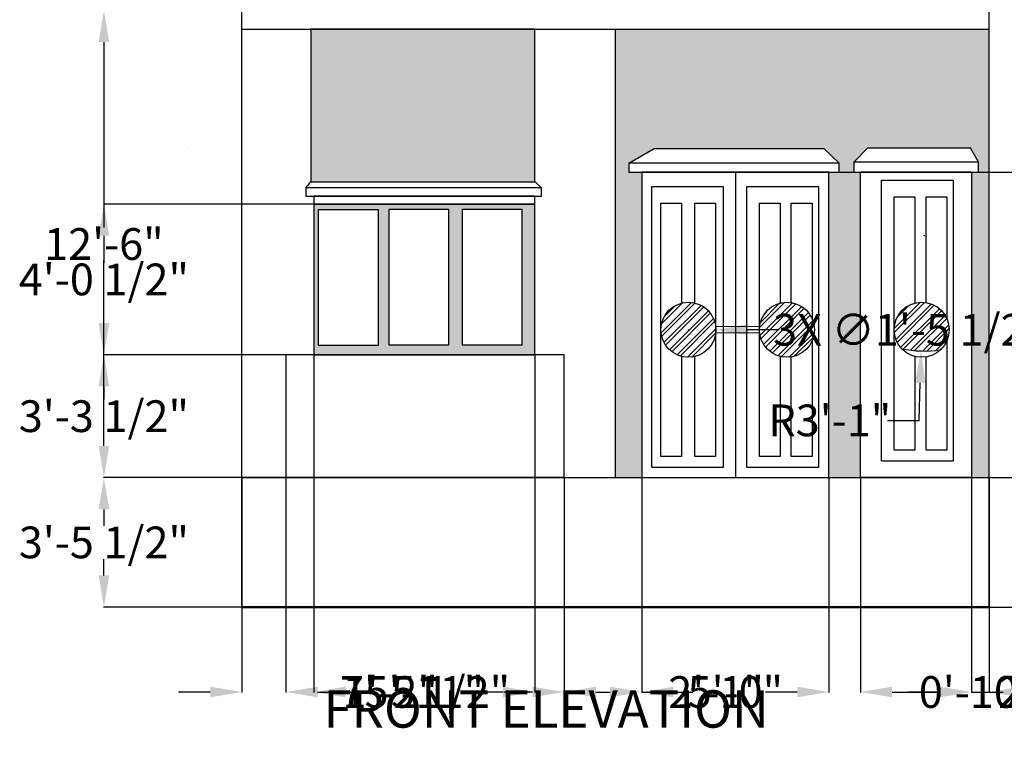
# Model space of a CAD drawing. Units: inches. Extents: x 21 to 3450, y 4 to 2137.
# Tile 5 of 14: x 2115 to 2431, y 1552 to 1783. Entities that reach past the tile are written whole.
import ezdxf

# ---------------------------------------------------------------- set-up
doc = ezdxf.new("R2010")
doc.units = ezdxf.units.IN
doc.header["$MEASUREMENT"] = 0
for name, color, linetype, lineweight in [('A-ANNO-DIMS', 2, 'Continuous', 18), ('A-ANNO-TEXT', 7, 'Continuous', 18), ('A-ELEV', 7, 'Continuous', 25), ('A-ELEV-PATT', 8, 'Continuous', 13), ('A-WALL', 7, 'Continuous', 50)]:
    doc.layers.add(name, color=color, linetype=linetype, lineweight=lineweight)
doc.styles.get("Standard").update_dxf_attribs({"font": 'arial.ttf'})
doc.dimstyles.get("Standard").update_dxf_attribs({"dimtxt": 10.18, "dimasz": 10.18, "dimexe": 0.18, "dimexo": 0.0625, "dimgap": 0.09, "dimtad": 0, "dimtih": 1, "dimtoh": 1, "dimdec": 0, "dimzin": 0, "dimdsep": 46, "dimlunit": 3, "dimtxsty": 'Standard', "dimcen": 0.09, "dimadec": 0, "dimazin": 0, "dimtfac": 1, "dimtdec": 0, "dimtofl": 0, "dimtmove": 0, "dimatfit": 3, "dimfxl": 1, "dimtolj": 1, "dimtzin": 0, "dimarcsym": 0})
pattern_1 = [(45, (255.9994, -6.4862), (-2.0417708, 2.0417708), []), (45, (257.3606, -6.4862), (-2.0417708, 2.0417708), [])]

# ---------------------------------------------------------------- blocks, each defined once
blk = doc.blocks.new('*D152')
at = {"layer": 'A-ANNO-DIMS', "color": 0, "lineweight": -2, "transparency": 16777216}
for p, q in [((2426.25, 2094.9), (2453.61, 2094.9)), ((2453.43, 2084.72), (2453.43, 1850.06)), ((2453.43, 1604.7), (2453.43, 1839.36)), ((2426.25, 1594.52), (2453.61, 1594.52))]:
    blk.add_line(p, q, dxfattribs=at)
at = {"layer": 'A-ANNO-DIMS', "color": 0, "transparency": 16777216}
for points in [[(2451.74, 2084.72), (2455.13, 2084.72), (2453.43, 2094.9)], [(2451.74, 1604.7), (2455.13, 1604.7), (2453.43, 1594.52)]]:
    blk.add_solid(points, dxfattribs=at)
at = {"layer": 'Defpoints', "color": 0, "transparency": 16777216}
for p in [(2426.18, 2094.9), (2453.43, 2094.9), (2426.18, 1594.52)]:
    blk.add_point(p, dxfattribs=at)
at = {"layer": 'A-ANNO-DIMS', "color": 0, "transparency": 16777216, "insert": (2453.43, 1844.71), "char_height": 10.18, "attachment_point": 5}
blk.add_mtext('\\A1;41\'-8 1/2"', dxfattribs=at)
blk = doc.blocks.new('*D153')
at = {"layer": 'A-ANNO-DIMS', "color": 0, "lineweight": -2, "transparency": 16777216}
for p, q in [((2186.12, 1636.08), (2141.7, 1636.08)), ((2141.88, 1625.9), (2141.88, 1620.66)), ((2141.88, 1604.7), (2141.88, 1609.94)), ((2186.12, 1594.52), (2141.7, 1594.52))]:
    blk.add_line(p, q, dxfattribs=at)
at = {"layer": 'A-ANNO-DIMS', "color": 0, "transparency": 16777216}
for points in [[(2140.19, 1625.9), (2143.58, 1625.9), (2141.88, 1636.08)], [(2140.19, 1604.7), (2143.58, 1604.7), (2141.88, 1594.52)]]:
    blk.add_solid(points, dxfattribs=at)
at = {"layer": 'Defpoints', "color": 0, "transparency": 16777216}
for p in [(2141.88, 1636.08), (2186.18, 1636.08), (2186.18, 1594.52)]:
    blk.add_point(p, dxfattribs=at)
at = {"layer": 'A-ANNO-DIMS', "color": 0, "transparency": 16777216, "insert": (2141.88, 1615.3), "char_height": 10.18, "attachment_point": 5}
blk.add_mtext('\\A1;3\'-5 1/2"', dxfattribs=at)
blk = doc.blocks.new('*D154')
at = {"layer": 'A-ANNO-DIMS', "color": 0, "lineweight": -2, "transparency": 16777216}
for p, q in [((2186.12, 1786.08), (2141.7, 1786.08)), ((2141.88, 1775.9), (2141.88, 1716.37)), ((2141.88, 1646.26), (2141.88, 1705.79)), ((2186.12, 1636.08), (2141.7, 1636.08))]:
    blk.add_line(p, q, dxfattribs=at)
at = {"layer": 'A-ANNO-DIMS', "color": 0, "transparency": 16777216}
for points in [[(2140.19, 1775.9), (2143.58, 1775.9), (2141.88, 1786.08)], [(2140.19, 1646.26), (2143.58, 1646.26), (2141.88, 1636.08)]]:
    blk.add_solid(points, dxfattribs=at)
at = {"layer": 'Defpoints', "color": 0, "transparency": 16777216}
for p in [(2141.88, 1786.08), (2186.18, 1786.08), (2186.18, 1636.08)]:
    blk.add_point(p, dxfattribs=at)
at = {"layer": 'A-ANNO-DIMS', "color": 0, "transparency": 16777216, "insert": (2141.88, 1711.08), "char_height": 10.18, "attachment_point": 5}
blk.add_mtext('\\A1;12\'-6"', dxfattribs=at)
blk = doc.blocks.new('*D161')
at = {"layer": 'A-ANNO-DIMS', "color": 0, "lineweight": -2, "transparency": 16777216}
for p, q in [((2186.18, 1636.02), (2186.18, 1567.09)), ((2200.32, 1636.02), (2200.32, 1567.09)), ((2176, 1567.27), (2165.82, 1567.27)), ((2210.5, 1567.27), (2220.68, 1567.27))]:
    blk.add_line(p, q, dxfattribs=at)
at = {"layer": 'A-ANNO-DIMS', "color": 0, "transparency": 16777216}
for points in [[(2176, 1568.97), (2176, 1565.57), (2186.18, 1567.27)], [(2210.5, 1568.97), (2210.5, 1565.57), (2200.32, 1567.27)]]:
    blk.add_solid(points, dxfattribs=at)
at = {"layer": 'Defpoints', "color": 0, "transparency": 16777216}
for p in [(2186.18, 1636.08), (2200.32, 1636.08), (2200.32, 1567.27)]:
    blk.add_point(p, dxfattribs=at)
at = {"layer": 'A-ANNO-DIMS', "color": 0, "transparency": 16777216, "insert": (2233.82, 1567.27), "char_height": 10.18, "attachment_point": 5}
blk.add_mtext('\\A1;1\'-2"', dxfattribs=at)
blk = doc.blocks.new('*D162')
at = {"layer": 'A-ANNO-DIMS', "color": 0, "lineweight": -2, "transparency": 16777216}
for p, q in [((2200.32, 1636.02), (2200.32, 1567.09)), ((2289.7, 1636.02), (2289.7, 1567.09)), ((2210.5, 1567.27), (2219.57, 1567.27)), ((2279.52, 1567.27), (2270.45, 1567.27))]:
    blk.add_line(p, q, dxfattribs=at)
at = {"layer": 'A-ANNO-DIMS', "color": 0, "transparency": 16777216}
for points in [[(2210.5, 1568.97), (2210.5, 1565.57), (2200.32, 1567.27)], [(2279.52, 1568.97), (2279.52, 1565.57), (2289.7, 1567.27)]]:
    blk.add_solid(points, dxfattribs=at)
at = {"layer": 'Defpoints', "color": 0, "transparency": 16777216}
for p in [(2200.32, 1636.08), (2289.7, 1636.08), (2289.7, 1567.27)]:
    blk.add_point(p, dxfattribs=at)
at = {"layer": 'A-ANNO-DIMS', "color": 0, "transparency": 16777216, "insert": (2245.01, 1567.27), "char_height": 10.18, "attachment_point": 5}
blk.add_mtext('\\A1;7\'-5 1/2"', dxfattribs=at)
blk = doc.blocks.new('*D163')
at = {"layer": 'A-ANNO-DIMS', "color": 0, "lineweight": -2, "transparency": 16777216}
for p, q in [((2289.7, 1636.02), (2289.7, 1567.09)), ((2314.57, 1636.02), (2314.57, 1567.09)), ((2299.88, 1567.27), (2304.39, 1567.27)), ((2314.57, 1567.27), (2324.75, 1567.27))]:
    blk.add_line(p, q, dxfattribs=at)
at = {"layer": 'A-ANNO-DIMS', "color": 0, "transparency": 16777216}
for points in [[(2299.88, 1568.97), (2299.88, 1565.57), (2289.7, 1567.27)], [(2304.39, 1568.97), (2304.39, 1565.57), (2314.57, 1567.27)]]:
    blk.add_solid(points, dxfattribs=at)
at = {"layer": 'Defpoints', "color": 0, "transparency": 16777216}
for p in [(2289.7, 1636.08), (2314.57, 1636.08), (2314.57, 1567.27)]:
    blk.add_point(p, dxfattribs=at)
at = {"layer": 'A-ANNO-DIMS', "color": 0, "transparency": 16777216, "insert": (2338.46, 1567.27), "char_height": 10.18, "attachment_point": 5}
blk.add_mtext('\\A1;2\'-1"', dxfattribs=at)
blk = doc.blocks.new('*D164')
at = {"layer": 'A-ANNO-DIMS', "color": 0, "lineweight": -2, "transparency": 16777216}
for p, q in [((2314.57, 1636.02), (2314.57, 1567.09)), ((2374.7, 1636.02), (2374.7, 1567.09)), ((2324.75, 1567.27), (2331.02, 1567.27)), ((2364.52, 1567.27), (2358.26, 1567.27))]:
    blk.add_line(p, q, dxfattribs=at)
at = {"layer": 'A-ANNO-DIMS', "color": 0, "transparency": 16777216}
for points in [[(2324.75, 1568.97), (2324.75, 1565.57), (2314.57, 1567.27)], [(2364.52, 1568.97), (2364.52, 1565.57), (2374.7, 1567.27)]]:
    blk.add_solid(points, dxfattribs=at)
at = {"layer": 'Defpoints', "color": 0, "transparency": 16777216}
for p in [(2314.57, 1636.08), (2374.7, 1636.08), (2374.7, 1567.27)]:
    blk.add_point(p, dxfattribs=at)
at = {"layer": 'A-ANNO-DIMS', "color": 0, "transparency": 16777216, "insert": (2344.64, 1567.27), "char_height": 10.18, "attachment_point": 5}
blk.add_mtext('\\A1;5\'-0"', dxfattribs=at)
blk = doc.blocks.new('*D165')
at = {"layer": 'A-ANNO-DIMS', "color": 0, "lineweight": -2, "transparency": 16777216}
for p, q in [((2374.7, 1636.02), (2374.7, 1567.09)), ((2384.8, 1636.02), (2384.8, 1567.09)), ((2364.52, 1567.27), (2354.34, 1567.27)), ((2394.98, 1567.27), (2405.16, 1567.27))]:
    blk.add_line(p, q, dxfattribs=at)
at = {"layer": 'A-ANNO-DIMS', "color": 0, "transparency": 16777216}
for points in [[(2364.52, 1568.97), (2364.52, 1565.57), (2374.7, 1567.27)], [(2394.98, 1568.97), (2394.98, 1565.57), (2384.8, 1567.27)]]:
    blk.add_solid(points, dxfattribs=at)
at = {"layer": 'Defpoints', "color": 0, "transparency": 16777216}
for p in [(2374.7, 1636.08), (2384.8, 1636.08), (2384.8, 1567.27)]:
    blk.add_point(p, dxfattribs=at)
at = {"layer": 'A-ANNO-DIMS', "color": 0, "transparency": 16777216, "insert": (2422.74, 1567.27), "char_height": 10.18, "attachment_point": 5}
blk.add_mtext('\\A1;0\'-10"', dxfattribs=at)
blk = doc.blocks.new('*D166')
at = {"layer": 'A-ANNO-DIMS', "color": 0, "lineweight": -2, "transparency": 16777216}
for p, q in [((2384.8, 1636.02), (2384.8, 1567.09)), ((2420.5, 1636.02), (2420.5, 1567.09)), ((2394.98, 1567.27), (2410.32, 1567.27)), ((2420.5, 1567.27), (2430.68, 1567.27))]:
    blk.add_line(p, q, dxfattribs=at)
at = {"layer": 'A-ANNO-DIMS', "color": 0, "transparency": 16777216}
for points in [[(2394.98, 1568.97), (2394.98, 1565.57), (2384.8, 1567.27)], [(2410.32, 1568.97), (2410.32, 1565.57), (2420.5, 1567.27)]]:
    blk.add_solid(points, dxfattribs=at)
at = {"layer": 'Defpoints', "color": 0, "transparency": 16777216}
for p in [(2384.8, 1636.08), (2420.5, 1636.08), (2420.5, 1567.27)]:
    blk.add_point(p, dxfattribs=at)
at = {"layer": 'A-ANNO-DIMS', "color": 0, "transparency": 16777216, "insert": (2460.2, 1567.27), "char_height": 10.18, "attachment_point": 5}
blk.add_mtext('\\A1;2\'-11 1/2"', dxfattribs=at)
blk = doc.blocks.new('*D167')
at = {"layer": 'A-ANNO-DIMS', "color": 0, "lineweight": -2, "transparency": 16777216}
for p, q in [((2420.5, 1636.02), (2420.5, 1567.09)), ((2426.18, 1636.02), (2426.18, 1567.09)), ((2410.32, 1567.27), (2400.14, 1567.27)), ((2436.36, 1567.27), (2446.54, 1567.27))]:
    blk.add_line(p, q, dxfattribs=at)
at = {"layer": 'A-ANNO-DIMS', "color": 0, "transparency": 16777216}
for points in [[(2410.32, 1568.97), (2410.32, 1565.57), (2420.5, 1567.27)], [(2436.36, 1568.97), (2436.36, 1565.57), (2426.18, 1567.27)]]:
    blk.add_solid(points, dxfattribs=at)
at = {"layer": 'Defpoints', "color": 0, "transparency": 16777216}
for p in [(2420.5, 1636.08), (2426.18, 1636.08), (2426.18, 1567.27)]:
    blk.add_point(p, dxfattribs=at)
at = {"layer": 'A-ANNO-DIMS', "color": 0, "transparency": 16777216, "insert": (2472.03, 1567.27), "char_height": 10.18, "attachment_point": 5}
blk.add_mtext('\\A1;0\'-5 1/2"', dxfattribs=at)
blk = doc.blocks.new('*D168')
at = {"layer": 'A-ANNO-DIMS', "color": 0, "lineweight": -2, "transparency": 16777216}
for p, q in [((2209.28, 1675.48), (2209.28, 1567.09)), ((2280.25, 1675.48), (2280.25, 1567.09)), ((2219.46, 1567.27), (2227.19, 1567.27)), ((2270.07, 1567.27), (2262.34, 1567.27))]:
    blk.add_line(p, q, dxfattribs=at)
at = {"layer": 'A-ANNO-DIMS', "color": 0, "transparency": 16777216}
for points in [[(2219.46, 1568.97), (2219.46, 1565.57), (2209.28, 1567.27)], [(2270.07, 1568.97), (2270.07, 1565.57), (2280.25, 1567.27)]]:
    blk.add_solid(points, dxfattribs=at)
at = {"layer": 'Defpoints', "color": 0, "transparency": 16777216}
for p in [(2209.28, 1675.54), (2280.25, 1675.54), (2280.25, 1567.27)]:
    blk.add_point(p, dxfattribs=at)
at = {"layer": 'A-ANNO-DIMS', "color": 0, "transparency": 16777216, "insert": (2244.76, 1567.27), "char_height": 10.18, "attachment_point": 5}
blk.add_mtext('\\A1;5\'-11"', dxfattribs=at)
blk = doc.blocks.new('*D169')
at = {"layer": 'A-ANNO-DIMS', "color": 0, "lineweight": -2, "transparency": 16777216}
for p, q in [((2280.19, 1723.89), (2141.7, 1723.89)), ((2141.88, 1713.71), (2141.88, 1705.07)), ((2141.88, 1685.72), (2141.88, 1694.36)), ((2280.19, 1675.54), (2141.7, 1675.54))]:
    blk.add_line(p, q, dxfattribs=at)
at = {"layer": 'A-ANNO-DIMS', "color": 0, "transparency": 16777216}
for points in [[(2140.19, 1713.71), (2143.58, 1713.71), (2141.88, 1723.89)], [(2140.19, 1685.72), (2143.58, 1685.72), (2141.88, 1675.54)]]:
    blk.add_solid(points, dxfattribs=at)
at = {"layer": 'Defpoints', "color": 0, "transparency": 16777216}
for p in [(2141.88, 1723.89), (2280.25, 1723.89), (2280.25, 1675.54)]:
    blk.add_point(p, dxfattribs=at)
at = {"layer": 'A-ANNO-DIMS', "color": 0, "transparency": 16777216, "insert": (2141.88, 1699.71), "char_height": 10.18, "attachment_point": 5}
blk.add_mtext('\\A1;4\'-0 1/2"', dxfattribs=at)
blk = doc.blocks.new('*D170')
at = {"layer": 'A-ANNO-DIMS', "color": 0, "lineweight": -2, "transparency": 16777216}
for p, q in [((2289.64, 1675.54), (2141.7, 1675.54)), ((2141.88, 1665.36), (2141.88, 1661.17)), ((2141.88, 1646.26), (2141.88, 1650.45)), ((2289.64, 1636.08), (2141.7, 1636.08))]:
    blk.add_line(p, q, dxfattribs=at)
at = {"layer": 'A-ANNO-DIMS', "color": 0, "transparency": 16777216}
for points in [[(2140.19, 1665.36), (2143.58, 1665.36), (2141.88, 1675.54)], [(2140.19, 1646.26), (2143.58, 1646.26), (2141.88, 1636.08)]]:
    blk.add_solid(points, dxfattribs=at)
at = {"layer": 'Defpoints', "color": 0, "transparency": 16777216}
for p in [(2141.88, 1675.54), (2289.7, 1675.54), (2289.7, 1636.08)]:
    blk.add_point(p, dxfattribs=at)
at = {"layer": 'A-ANNO-DIMS', "color": 0, "transparency": 16777216, "insert": (2141.88, 1655.81), "char_height": 10.18, "attachment_point": 5}
blk.add_mtext('\\A1;3\'-3 1/2"', dxfattribs=at)
blk = doc.blocks.new('*D173')
at = {"layer": 'A-ANNO-DIMS', "color": 0, "lineweight": -2, "transparency": 16777216}
for p, q in [((2374.76, 1734.1), (2453.61, 1734.1)), ((2453.43, 1723.92), (2453.43, 1690.38)), ((2453.43, 1646.26), (2453.43, 1679.8)), ((2374.76, 1636.08), (2453.61, 1636.08))]:
    blk.add_line(p, q, dxfattribs=at)
at = {"layer": 'A-ANNO-DIMS', "color": 0, "transparency": 16777216}
for points in [[(2451.74, 1723.92), (2455.13, 1723.92), (2453.43, 1734.1)], [(2451.74, 1646.26), (2455.13, 1646.26), (2453.43, 1636.08)]]:
    blk.add_solid(points, dxfattribs=at)
at = {"layer": 'Defpoints', "color": 0, "transparency": 16777216}
for p in [(2374.7, 1734.1), (2453.43, 1734.1), (2374.7, 1636.08)]:
    blk.add_point(p, dxfattribs=at)
at = {"layer": 'A-ANNO-DIMS', "color": 0, "transparency": 16777216, "insert": (2453.43, 1685.09), "char_height": 10.18, "attachment_point": 5}
blk.add_mtext('\\A1;8\'-2"', dxfattribs=at)
blk = doc.blocks.new('*D195')
at = {"layer": 'A-ANNO-DIMS', "color": 0, "lineweight": -2, "transparency": 16777216}
for p, q in [((2329.47, 1683.55), (2329.65, 1683.55)), ((2329.56, 1683.46), (2329.56, 1683.64)), ((2358.76, 1683.55), (2348.58, 1683.55))]:
    blk.add_line(p, q, dxfattribs=at)
at = {"layer": 'A-ANNO-DIMS', "color": 0, "transparency": 16777216}
blk.add_solid([(2348.58, 1685.25), (2348.58, 1681.85), (2338.4, 1683.55)], dxfattribs=at)
at = {"layer": 'Defpoints', "color": 0, "transparency": 16777216}
for p in [(2320.73, 1683.55), (2338.4, 1683.55)]:
    blk.add_point(p, dxfattribs=at)
at = {"layer": 'A-ANNO-DIMS', "color": 0, "transparency": 16777216, "insert": (2400.44, 1683.55), "char_height": 10.18, "attachment_point": 5}
blk.add_mtext('\\A1;3X ∅1\'-5 1/2"', dxfattribs=at)
blk = doc.blocks.new('*D196')
at = {"layer": 'A-ANNO-DIMS', "color": 0, "lineweight": -2, "transparency": 16777216}
for p, q in [((2405.24, 1713.84), (2405.42, 1713.84)), ((2405.33, 1713.75), (2405.33, 1713.93)), ((2403.63, 1654.47), (2403.97, 1666.56)), ((2393.45, 1654.47), (2403.63, 1654.47))]:
    blk.add_line(p, q, dxfattribs=at)
at = {"layer": 'A-ANNO-DIMS', "color": 0, "transparency": 16777216}
blk.add_solid([(2402.28, 1666.61), (2405.67, 1666.51), (2404.27, 1676.74)], dxfattribs=at)
at = {"layer": 'Defpoints', "color": 0, "transparency": 16777216}
for p in [(2405.33, 1713.84), (2404.27, 1676.74)]:
    blk.add_point(p, dxfattribs=at)
at = {"layer": 'A-ANNO-DIMS', "color": 0, "transparency": 16777216, "insert": (2374.95, 1654.47), "char_height": 10.18, "attachment_point": 5}
blk.add_mtext('\\A1;R3\'-1"', dxfattribs=at)

msp = doc.modelspace()

# ---------------------------------------------------------------- hatches: boundary and pattern name
at = {"layer": 'A-ELEV-PATT'}
h = msp.add_hatch(dxfattribs=at)
h.set_pattern_fill('AR-BRELM', color=256, scale=1.9)
h.set_pattern_definition([(0, (0, 0), (0, 10.1346), [14.4875, -0.7125]), (0, (0, 4.275), (0, 10.1346), [14.4875, -0.7125]), (0, (3.8, 5.067), (0, 10.1346), [6.8875, -0.7125]), (0, (3.8, 9.342), (0, 10.1346), [6.8875, -0.7125]), (90, (0, 0), (-15.2, 9e-16), [4.275, -5.8596]), (90, (-0.713, 0), (-15.2, 9e-16), [4.275, -5.8596]), (90, (3.8, 5.067), (-7.6, 5e-16), [4.275, -5.8596]), (90, (3.0875, 5.067), (-7.6, 5e-16), [4.275, -5.8596])])
h.paths.add_polyline_path([(2282.59, 1918.08), (2210.89, 1918.08), (2210.89, 1885.65), (2282.59, 1885.65)])
h.paths.add_polyline_path([(2280.2, 1780.08), (2208.3, 1780.08), (2208.3, 1731.04), (2280.2, 1731.04)])
h.paths.add_polyline_path([(2350.36, 1918.08), (2306.18, 1918.08), (2306.18, 1829.6), (2319, 1829.6), (2319, 1875.89), (2350.36, 1875.89)])
h.paths.add_polyline_path([(2426.18, 1780.08), (2306.18, 1780.08), (2306.18, 1636.08), (2314.57, 1636.08), (2314.57, 1734.1), (2310.48, 1734.1), (2310.48, 1737.04), (2318.62, 1741.75), (2373, 1741.75), (2378.02, 1737.04), (2378.02, 1734.1), (2374.7, 1734.1), (2374.7, 1636.08), (2384.8, 1636.08), (2384.8, 1734.1), (2382.71, 1734.1), (2382.71, 1737.37), (2387.22, 1741.92), (2420.14, 1741.92), (2422.71, 1737.37), (2422.71, 1734.1), (2420.5, 1734.1), (2420.5, 1636.08), (2426.18, 1636.08)])
h.paths.add_polyline_path([(2426.18, 2055.62), (2306.18, 2055.62), (2306.18, 1977.49), (2426.18, 1977.49)])
h = msp.add_hatch(color=256, dxfattribs=at)
h.dxf.hatch_style = 1
h.paths.add_polyline_path([(2209.28, 1723.89), (2209.28, 1675.54), (2280.25, 1675.54), (2280.25, 1723.89)])
h.paths.add_polyline_path([(2233.43, 1722.27), (2252.56, 1722.27), (2252.56, 1678.62), (2233.43, 1678.62)], flags=16)
h.paths.add_polyline_path([(2229.92, 1678.52), (2210.79, 1678.52), (2210.79, 1722.17), (2229.92, 1722.17)], flags=16)
h.paths.add_polyline_path([(2257, 1722.27), (2276.13, 1722.27), (2276.13, 1678.62), (2257, 1678.62)], flags=16)
h = msp.add_hatch(dxfattribs=at)
h.set_pattern_fill('ANSI32', color=256, scale=7.7)
h.set_pattern_definition(pattern_1)
h.paths.add_polyline_path([(2320.73, 1683.55, 0.927615), (2338.3, 1682.23), (2338.3, 1684.87, 0.927615)])
h.paths.add_polyline_path([(2352.35, 1683.55, 1), (2370.03, 1683.55, 1)])
h = msp.add_hatch(dxfattribs=at)
h.set_pattern_fill('ANSI32', color=256, scale=7.7)
h.set_pattern_definition(pattern_1)
h.paths.add_polyline_path([(2410.48, 1677.08, 0.208441), (2413.3, 1683.55, 1), (2395.62, 1683.55, 0.193508), (2398.08, 1677.44, 0.084081)])

# ---------------------------------------------------------------- linework, layer by layer
at = {"layer": 'A-ELEV'}
for p, q in [((2186.18, 1594.52), (2186.18, 1977.49)), ((2426.18, 1594.52), (2426.18, 1977.49)), ((2186.18, 1780.08), (2426.18, 1780.08)), ((2306.18, 1636.08), (2306.18, 1780.08)), ((2310.48, 1737.04), (2318.62, 1741.75)), ((2318.62, 1741.75), (2373, 1741.75)), ((2378.02, 1737.04), (2373, 1741.75)), ((2382.71, 1737.37), (2387.22, 1741.92)), ((2387.22, 1741.92), (2420.14, 1741.92)), ((2422.71, 1737.37), (2420.14, 1741.92)), ((2344.64, 1734.1), (2344.64, 1636.08)), ((2206.72, 1729.16), (2208.3, 1731.04)), ((2208.3, 1731.04), (2280.32, 1731.04)), ((2282.39, 1729.16), (2280.32, 1731.04)), ((2338.29, 1682.72), (2352.34, 1682.55)), ((2338.31, 1684.72), (2352.37, 1684.55)), ((2186.18, 1636.08), (2426.18, 1636.08))]:
    msp.add_line(p, q, dxfattribs=at)
for points in [[(2208.3, 1731.04), (2208.3, 1731.04), (2280.2, 1731.04), (2280.2, 1731.04), (2280.2, 1780.08), (2280.2, 1780.08), (2208.3, 1780.08), (2208.3, 1780.08)], [(2169.13, 1742.01), (2169.13, 1742.01)], [(2310.48, 1734.1), (2310.48, 1734.1), (2378.02, 1734.1), (2378.02, 1734.1), (2378.02, 1737.04), (2378.02, 1737.04), (2310.48, 1737.04), (2310.48, 1737.04)], [(2382.71, 1734.1), (2382.71, 1734.1), (2422.71, 1734.1), (2422.71, 1734.1), (2422.71, 1737.37), (2422.71, 1737.37), (2382.71, 1737.37), (2382.71, 1737.37)], [(2314.57, 1636.08), (2314.57, 1636.08), (2374.7, 1636.08), (2374.7, 1636.08), (2374.7, 1734.1), (2374.7, 1734.1), (2314.57, 1734.1), (2314.57, 1734.1)], [(2384.8, 1734.1), (2384.8, 1734.1), (2420.5, 1734.1), (2420.5, 1734.1), (2420.5, 1734.1), (2420.5, 1734.1), (2384.8, 1734.1), (2384.8, 1734.1)], [(2317.78, 1729.56), (2317.78, 1729.56), (2340.75, 1729.56), (2340.75, 1729.56), (2340.75, 1639.33), (2340.75, 1639.33), (2317.78, 1639.33), (2317.78, 1639.33)], [(2348.34, 1729.56), (2348.34, 1729.56), (2371.31, 1729.56), (2371.31, 1729.56), (2371.31, 1639.33), (2371.31, 1639.33), (2348.34, 1639.33), (2348.34, 1639.33)], [(2391.61, 1731.59), (2391.61, 1731.59), (2414.58, 1731.59), (2414.58, 1731.59), (2414.58, 1641.37), (2414.58, 1641.37), (2391.61, 1641.37), (2391.61, 1641.37)], [(2206.72, 1726.48), (2206.72, 1726.48), (2282.39, 1726.48), (2282.39, 1726.48), (2282.39, 1729.16), (2282.39, 1729.16), (2206.72, 1729.16), (2206.72, 1729.16)], [(2209.28, 1723.89), (2209.28, 1723.89), (2280.2, 1723.89), (2280.2, 1723.89), (2280.2, 1726.48), (2280.2, 1726.48), (2209.28, 1726.48), (2209.28, 1726.48)], [(2209.28, 1675.54), (2209.28, 1675.54), (2280.25, 1675.54), (2280.25, 1675.54), (2280.25, 1723.89), (2280.25, 1723.89), (2209.28, 1723.89), (2209.28, 1723.89)], [(2210.79, 1722.17), (2210.79, 1722.17), (2229.92, 1722.17), (2229.92, 1722.17), (2229.92, 1678.52), (2229.92, 1678.52), (2210.79, 1678.52), (2210.79, 1678.52)], [(2233.43, 1722.27), (2233.43, 1722.27), (2252.56, 1722.27), (2252.56, 1722.27), (2252.56, 1678.62), (2252.56, 1678.62), (2233.43, 1678.62), (2233.43, 1678.62)], [(2257, 1722.27), (2257, 1722.27), (2276.13, 1722.27), (2276.13, 1722.27), (2276.13, 1678.62), (2276.13, 1678.62), (2257, 1678.62), (2257, 1678.62)], [(2200.32, 1636.08), (2200.32, 1636.08), (2289.7, 1636.08), (2289.7, 1636.08), (2289.7, 1675.54), (2289.7, 1675.54), (2200.32, 1675.54), (2200.32, 1675.54)]]:
    msp.add_lwpolyline(points, close=True, dxfattribs=at)
for points in [[(2420.5, 1734.1), (2420.5, 1636.08), (2420.5, 1636.08), (2384.8, 1636.08), (2384.8, 1636.08), (2384.8, 1734.1)], [(2327.37, 1674.99), (2327.37, 1642.9), (2327.37, 1642.9), (2320.68, 1642.9), (2320.68, 1642.9), (2320.68, 1724.21), (2320.68, 1724.21), (2327.37, 1724.21), (2327.37, 1724.21), (2327.37, 1692.11)], [(2331.61, 1692.15), (2331.61, 1724.21), (2331.61, 1724.21), (2338.3, 1724.21), (2338.3, 1724.21), (2338.3, 1642.9), (2338.3, 1642.9), (2331.61, 1642.9), (2331.61, 1642.9), (2331.61, 1674.96)], [(2359.04, 1674.98), (2359.04, 1642.9), (2359.04, 1642.9), (2352.35, 1642.9), (2352.35, 1642.9), (2352.35, 1724.21), (2352.35, 1724.21), (2359.04, 1724.21), (2359.04, 1724.21), (2359.04, 1692.12)], [(2362.61, 1692.27), (2362.61, 1724.21), (2362.61, 1724.21), (2369.31, 1724.21), (2369.31, 1724.21), (2369.31, 1687.05)], [(2402.32, 1674.98), (2402.32, 1644.93), (2402.32, 1644.93), (2395.62, 1644.93), (2395.62, 1644.93), (2395.62, 1726.25), (2395.62, 1726.25), (2402.32, 1726.25), (2402.32, 1726.25), (2402.32, 1692.12)], [(2405.88, 1692.27), (2405.88, 1726.25), (2405.88, 1726.25), (2412.58, 1726.25), (2412.58, 1726.25), (2412.58, 1687.05)], [(2369.31, 1680.06), (2369.31, 1642.9), (2369.31, 1642.9), (2362.61, 1642.9), (2362.61, 1642.9), (2362.61, 1674.83)], [(2412.58, 1680.06), (2412.58, 1644.93), (2412.58, 1644.93), (2405.88, 1644.93), (2405.88, 1644.93), (2405.88, 1674.83)]]:
    msp.add_lwpolyline(points, dxfattribs=at)
for centre in [(2329.56, 1683.55), (2361.19, 1683.55), (2404.46, 1683.55)]:
    msp.add_circle(centre, 8.84, dxfattribs=at)
msp.add_arc((2405.33, 1713.84), 37.12, 258.7429, 277.9677, dxfattribs=at)
at = {"layer": 'A-WALL'}
msp.add_line((2186.18, 1594.52), (2426.18, 1594.52), dxfattribs=at)

# ---------------------------------------------------------------- texts
at = {"layer": 'A-ANNO-TEXT', "insert": (2212.38, 1567.82), "char_height": 12, "attachment_point": 1}
msp.add_mtext_dynamic_manual_height_columns('FRONT ELEVATION', width=266.8546, gutter_width=1, heights=[0], dxfattribs=at)

# ---------------------------------------------------------------- dimensions: what is measured, and where the dimension line sits
at = {"layer": 'A-ANNO-DIMS'}
for base, p1, p2, picture, middle in [((2453.43, 2094.9), (2426.18, 1594.52), (2426.18, 2094.9), '*D152', (2453.43, 1844.71)), ((2141.88, 1786.08), (2186.18, 1636.08), (2186.18, 1786.08), '*D154', (2141.88, 1711.08)), ((2453.43, 1734.1), (2374.7, 1636.08), (2374.7, 1734.1), '*D173', (2453.43, 1685.09)), ((2141.883763, 1723.889586), (2280.251024, 1675.539595), (2280.251024, 1723.889586), '*D169', (2141.883763, 1699.71459)), ((2141.88, 1675.54), (2289.7, 1636.08), (2289.7, 1675.54), '*D170', (2141.88, 1655.81)), ((2141.88, 1636.08), (2186.18, 1594.52), (2186.18, 1636.08), '*D153', (2141.88, 1615.3))]:
    dim = msp.add_linear_dim(base=base, p1=p1, p2=p2, angle=90, dimstyle='Standard', override={"dimdec": 1, "dimlfac": 1, "dimrnd": 0, "dimzin": 1, "dimdsep": 46, "dimlunit": 4, "dimfrac": 2}, dxfattribs=at)
    dim.commit()
    dim.dimension.update_dxf_attribs({"geometry": picture, "text_midpoint": middle})
dim = msp.add_radius_dim(center=(2405.33, 1713.84), mpoint=(2404.27, 1676.74), dimstyle='Standard', override={"dimdec": 1, "dimlfac": 1, "dimrnd": 0, "dimzin": 1, "dimdsep": 46, "dimlunit": 4, "dimfrac": 2}, dxfattribs=at)
dim.commit()
dim.dimension.update_dxf_attribs({"geometry": '*D196', "text_midpoint": (2374.95, 1654.47), "dimtype": 164})
dim = msp.add_diameter_dim_2p(p1=(2320.73, 1683.55), p2=(2338.4, 1683.55), text='3X <>', dimstyle='Standard', override={"dimdec": 1, "dimlfac": 1, "dimrnd": 0, "dimzin": 1, "dimdsep": 46, "dimlunit": 4, "dimfrac": 2}, dxfattribs=at)
dim.commit()
dim.dimension.update_dxf_attribs({"geometry": '*D195', "text_midpoint": (2358.76, 1683.55), "dimtype": 163})
for base, p1, p2, picture, middle in [((2280.25, 1567.27), (2209.28, 1675.54), (2280.25, 1675.54), '*D168', (2244.76, 1567.27)), ((2200.32, 1567.27), (2186.18, 1636.08), (2200.32, 1636.08), '*D161', (2233.82, 1567.27)), ((2289.7, 1567.27), (2200.32, 1636.08), (2289.7, 1636.08), '*D162', (2245.01, 1567.27)), ((2314.57, 1567.27), (2289.7, 1636.08), (2314.57, 1636.08), '*D163', (2338.46, 1567.27)), ((2374.7, 1567.27), (2314.57, 1636.08), (2374.7, 1636.08), '*D164', (2344.64, 1567.27)), ((2384.8, 1567.27), (2374.7, 1636.08), (2384.8, 1636.08), '*D165', (2422.74, 1567.27)), ((2420.5, 1567.27), (2384.8, 1636.08), (2420.5, 1636.08), '*D166', (2460.2, 1567.27)), ((2426.18, 1567.27), (2420.5, 1636.08), (2426.18, 1636.08), '*D167', (2472.03, 1567.27))]:
    dim = msp.add_linear_dim(base=base, p1=p1, p2=p2, dimstyle='Standard', override={"dimdec": 1, "dimlfac": 1, "dimrnd": 0, "dimzin": 1, "dimdsep": 46, "dimlunit": 4, "dimfrac": 2}, dxfattribs=at)
    dim.commit()
    dim.dimension.update_dxf_attribs({"geometry": picture, "text_midpoint": middle})

doc.saveas('drawing.dxf')
